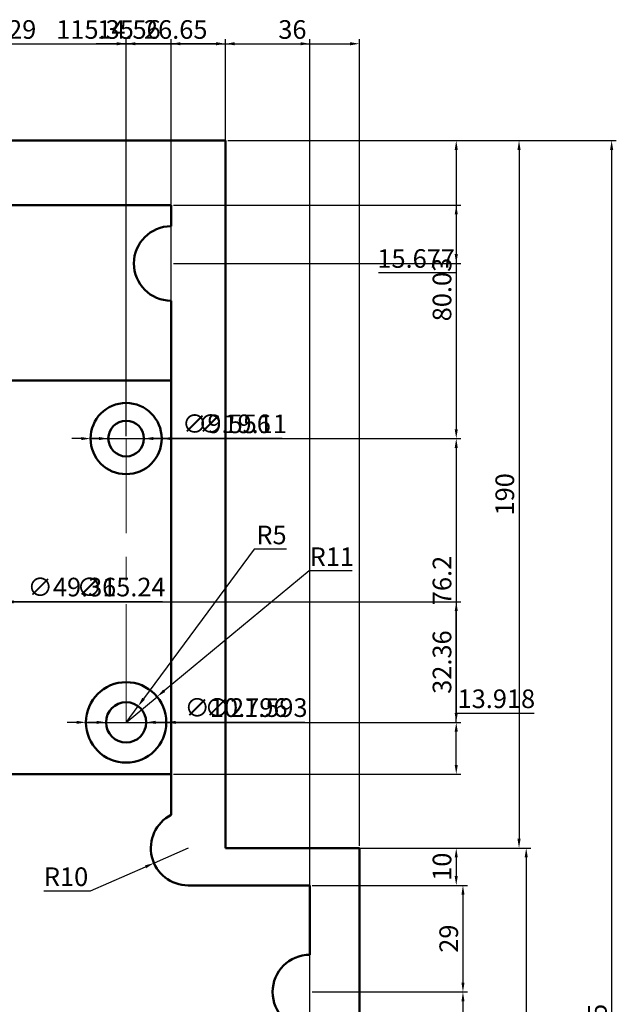
# Model space of a CAD drawing. Units: millimetres. Extents: x 1744 to 2162, y 1763 to 2334.
# Tile 5 of 5: x 1975 to 2135, y 2070 to 2334. Entities that reach past the tile are written whole.
import ezdxf

# ---------------------------------------------------------------- set-up
doc = ezdxf.new("R2010")
doc.units = ezdxf.units.MM
doc.linetypes.add('CENTER', pattern=[50.8, 31.75, -6.35, 6.35, -6.35])
for name, color, linetype, lineweight in [('M-CNTR', 4, 'CENTER', 18), ('M-DIMS', 2, 'Continuous', 25), ('M-OUTL', 7, 'Continuous', 50)]:
    doc.layers.add(name, color=color, linetype=linetype, lineweight=lineweight)
doc.styles.get("Standard").update_dxf_attribs({"font": 'arial.ttf'})
doc.dimstyles.new('ISO-25', dxfattribs={"dimtxt": 5, "dimasz": 2.5, "dimexe": 1.25, "dimexo": 0.625, "dimtad": 1, "dimtoh": 1, "dimdec": 0, "dimtxsty": 'Standard', "dimcen": 2.5, "dimadec": 0, "dimazin": 0, "dimtfac": 1, "dimtdec": 0, "dimtmove": 0, "dimatfit": 3, "dimfxl": 1, "dimarcsym": 0})

# ---------------------------------------------------------------- blocks, each defined once
blk = doc.blocks.new('*D2')
at = {"layer": 'Defpoints', "color": 0, "transparency": 16777216}
for p in [(2029.83, 2301.76), (2035.83, 1826.76), (2133.56, 1826.76)]:
    blk.add_point(p, dxfattribs=at)
at = {"layer": 'M-DIMS', "color": 0, "lineweight": -2, "transparency": 16777216}
for p, q in [((2030.45, 2301.76), (2134.81, 2301.76)), ((2133.56, 2299.26), (2133.56, 1829.26)), ((2036.45, 1826.76), (2134.81, 1826.76))]:
    blk.add_line(p, q, dxfattribs=at)
at = {"layer": 'M-DIMS', "color": 0, "transparency": 16777216}
for points in [[(2133.14, 2299.26), (2133.98, 2299.26), (2133.56, 2301.76)], [(2133.14, 1829.26), (2133.98, 1829.26), (2133.56, 1826.76)]]:
    blk.add_solid(points, dxfattribs=at)
at = {"layer": 'M-DIMS', "color": 0, "transparency": 16777216, "insert": (2130.39, 2064.26), "char_height": 5, "attachment_point": 5, "rotation": 90}
blk.add_mtext('475', dxfattribs=at)
blk = doc.blocks.new('*D3')
at = {"layer": 'Defpoints', "color": 0, "transparency": 16777216}
for p in [(2029.83, 2301.76), (2029.83, 2111.76), (2108.69, 2111.76)]:
    blk.add_point(p, dxfattribs=at)
at = {"layer": 'M-DIMS', "color": 0, "lineweight": -2, "transparency": 16777216}
for p, q in [((2030.45, 2301.76), (2109.94, 2301.76)), ((2108.69, 2299.26), (2108.69, 2114.26)), ((2030.45, 2111.76), (2109.94, 2111.76))]:
    blk.add_line(p, q, dxfattribs=at)
at = {"layer": 'M-DIMS', "color": 0, "transparency": 16777216}
for points in [[(2108.27, 2299.26), (2109.1, 2299.26), (2108.69, 2301.76)], [(2108.27, 2114.26), (2109.1, 2114.26), (2108.69, 2111.76)]]:
    blk.add_solid(points, dxfattribs=at)
at = {"layer": 'M-DIMS', "color": 0, "transparency": 16777216, "insert": (2105.51, 2206.76), "char_height": 5, "attachment_point": 5, "rotation": 90}
blk.add_mtext('190', dxfattribs=at)
blk = doc.blocks.new('*D4')
at = {"layer": 'Defpoints', "color": 0, "transparency": 16777216}
for p in [(2065.83, 2111.76), (2065.83, 1844.08), (2110.62, 1844.08)]:
    blk.add_point(p, dxfattribs=at)
at = {"layer": 'M-DIMS', "color": 0, "lineweight": -2, "transparency": 16777216}
for p, q in [((2066.45, 2111.76), (2111.87, 2111.76)), ((2110.62, 2109.26), (2110.62, 1846.58)), ((2066.45, 1844.08), (2111.87, 1844.08))]:
    blk.add_line(p, q, dxfattribs=at)
at = {"layer": 'M-DIMS', "color": 0, "transparency": 16777216}
for points in [[(2110.2, 2109.26), (2111.04, 2109.26), (2110.62, 2111.76)], [(2110.2, 1846.58), (2111.04, 1846.58), (2110.62, 1844.08)]]:
    blk.add_solid(points, dxfattribs=at)
at = {"layer": 'M-DIMS', "color": 0, "transparency": 16777216, "insert": (2107.44, 1977.92), "char_height": 5, "attachment_point": 5, "rotation": 90}
blk.add_mtext('268', dxfattribs=at)
blk = doc.blocks.new('*D21')
at = {"layer": 'Defpoints', "color": 0, "transparency": 16777216}
for p in [(2019.83, 2111.76), (2010.67, 2107.74)]:
    blk.add_point(p, dxfattribs=at)
at = {"layer": 'M-DIMS', "color": 0, "lineweight": -2, "transparency": 16777216}
for p, q in [((2019.83, 2111.76), (2010.67, 2107.74)), ((1993.64, 2100.25), (2008.38, 2106.73)), ((1981.09, 2100.25), (1993.64, 2100.25))]:
    blk.add_line(p, q, dxfattribs=at)
at = {"layer": 'M-DIMS', "color": 0, "transparency": 16777216}
blk.add_solid([(2008.21, 2107.11), (2008.55, 2106.35), (2010.67, 2107.74)], dxfattribs=at)
at = {"layer": 'M-DIMS', "color": 0, "transparency": 16777216, "insert": (1987.05, 2103.43), "char_height": 5, "attachment_point": 5}
blk.add_mtext('R10', dxfattribs=at)
blk = doc.blocks.new('*D22')
at = {"layer": 'Defpoints', "color": 0, "transparency": 16777216}
for p in [(2011.49, 2152.42), (2003.18, 2145.53)]:
    blk.add_point(p, dxfattribs=at)
at = {"layer": 'M-DIMS', "color": 0, "lineweight": -2, "transparency": 16777216}
for p, q in [((2052.3, 2186.23), (2013.42, 2154.01)), ((2063.91, 2186.23), (2052.3, 2186.23)), ((2003.18, 2145.53), (2011.49, 2152.42))]:
    blk.add_line(p, q, dxfattribs=at)
at = {"layer": 'M-DIMS', "color": 0, "transparency": 16777216}
blk.add_solid([(2013.15, 2154.33), (2013.68, 2153.69), (2011.49, 2152.42)], dxfattribs=at)
at = {"layer": 'M-DIMS', "color": 0, "transparency": 16777216, "insert": (2058.42, 2189.36), "char_height": 5, "attachment_point": 5}
blk.add_mtext('R11', dxfattribs=at)
blk = doc.blocks.new('*D23')
at = {"layer": 'Defpoints', "color": 0, "transparency": 16777216}
for p in [(2006.39, 2149.87), (2003.18, 2145.53)]:
    blk.add_point(p, dxfattribs=at)
at = {"layer": 'M-DIMS', "color": 0, "lineweight": -2, "transparency": 16777216}
for p, q in [((2037.53, 2192.04), (2007.87, 2151.88)), ((2046.26, 2192.04), (2037.53, 2192.04)), ((2003.18, 2145.53), (2006.39, 2149.87))]:
    blk.add_line(p, q, dxfattribs=at)
at = {"layer": 'M-DIMS', "color": 0, "transparency": 16777216}
blk.add_solid([(2007.54, 2152.13), (2008.21, 2151.63), (2006.39, 2149.87)], dxfattribs=at)
at = {"layer": 'M-DIMS', "color": 0, "transparency": 16777216, "insert": (2042.21, 2195.21), "char_height": 5, "attachment_point": 5}
blk.add_mtext('R5', dxfattribs=at)
blk = doc.blocks.new('*D24')
at = {"layer": 'Defpoints', "color": 0, "transparency": 16777216}
for p in [(2052.51, 2101.76), (2052.51, 2073.12), (2093.63, 2073.12)]:
    blk.add_point(p, dxfattribs=at)
at = {"layer": 'M-DIMS', "color": 0, "lineweight": -2, "transparency": 16777216}
for p, q in [((2053.13, 2101.76), (2094.88, 2101.76)), ((2093.63, 2099.26), (2093.63, 2075.62)), ((2053.13, 2073.12), (2094.88, 2073.12))]:
    blk.add_line(p, q, dxfattribs=at)
at = {"layer": 'M-DIMS', "color": 0, "transparency": 16777216}
for points in [[(2093.22, 2099.26), (2094.05, 2099.26), (2093.63, 2101.76)], [(2093.22, 2075.62), (2094.05, 2075.62), (2093.63, 2073.12)]]:
    blk.add_solid(points, dxfattribs=at)
at = {"layer": 'M-DIMS', "color": 0, "transparency": 16777216, "insert": (2090.46, 2087.44), "char_height": 5, "attachment_point": 5, "rotation": 90}
blk.add_mtext('29', dxfattribs=at)
blk = doc.blocks.new('*D25')
at = {"layer": 'Defpoints', "color": 0, "transparency": 16777216}
for p in [(2052.51, 2073.12), (2052.51, 1966.98), (2093.63, 1966.98)]:
    blk.add_point(p, dxfattribs=at)
at = {"layer": 'M-DIMS', "color": 0, "lineweight": -2, "transparency": 16777216}
for p, q in [((2053.13, 2073.12), (2094.88, 2073.12)), ((2093.63, 2070.62), (2093.63, 1969.48)), ((2053.13, 1966.98), (2094.88, 1966.98))]:
    blk.add_line(p, q, dxfattribs=at)
at = {"layer": 'M-DIMS', "color": 0, "transparency": 16777216}
for points in [[(2093.22, 2070.62), (2094.05, 2070.62), (2093.63, 2073.12)], [(2093.22, 1969.48), (2094.05, 1969.48), (2093.63, 1966.98)]]:
    blk.add_solid(points, dxfattribs=at)
at = {"layer": 'M-DIMS', "color": 0, "transparency": 16777216, "insert": (2090.46, 2020.05), "char_height": 5, "attachment_point": 5, "rotation": 90}
blk.add_mtext('106', dxfattribs=at)
blk = doc.blocks.new('*D29')
at = {"layer": 'Defpoints', "color": 0, "transparency": 16777216}
for p in [(2052.51, 2327.76), (2052.51, 1966.98), (1937.15, 1938.72)]:
    blk.add_point(p, dxfattribs=at)
at = {"layer": 'M-DIMS', "color": 0, "lineweight": -2, "transparency": 16777216}
for p, q in [((1937.15, 1939.34), (1937.15, 2329.01)), ((1939.65, 2327.76), (2050.01, 2327.76)), ((2052.51, 1967.6), (2052.51, 2329.01))]:
    blk.add_line(p, q, dxfattribs=at)
at = {"layer": 'M-DIMS', "color": 0, "transparency": 16777216}
for points in [[(1939.65, 2328.18), (1939.65, 2327.34), (1937.15, 2327.76)], [(2050.01, 2328.18), (2050.01, 2327.34), (2052.51, 2327.76)]]:
    blk.add_solid(points, dxfattribs=at)
at = {"layer": 'M-DIMS', "color": 0, "transparency": 16777216, "insert": (1994.83, 2330.94), "char_height": 5, "attachment_point": 5}
blk.add_mtext('115.35', dxfattribs=at)
blk = doc.blocks.new('*D34')
at = {"layer": 'Defpoints', "color": 0, "transparency": 16777216}
for p in [(2003.18, 2327.76), (2003.18, 2221.73), (1937.89, 2177.89)]:
    blk.add_point(p, dxfattribs=at)
at = {"layer": 'M-DIMS', "color": 0, "lineweight": -2, "transparency": 16777216}
for p, q in [((1937.89, 2178.51), (1937.89, 2329.01)), ((1940.39, 2327.76), (2000.68, 2327.76)), ((2003.18, 2222.36), (2003.18, 2329.01))]:
    blk.add_line(p, q, dxfattribs=at)
at = {"layer": 'M-DIMS', "color": 0, "transparency": 16777216}
for points in [[(1940.39, 2328.18), (1940.39, 2327.34), (1937.89, 2327.76)], [(2000.68, 2328.18), (2000.68, 2327.34), (2003.18, 2327.76)]]:
    blk.add_solid(points, dxfattribs=at)
at = {"layer": 'M-DIMS', "color": 0, "transparency": 16777216, "insert": (1970.53, 2330.94), "char_height": 5, "attachment_point": 5}
blk.add_mtext('65.29', dxfattribs=at)
blk = doc.blocks.new('*D35')
at = {"layer": 'Defpoints', "color": 0, "transparency": 16777216}
for p in [(2003.18, 2327.76), (2029.83, 2301.76), (2003.18, 2221.73)]:
    blk.add_point(p, dxfattribs=at)
at = {"layer": 'M-DIMS', "color": 0, "lineweight": -2, "transparency": 16777216}
for p, q in [((2003.18, 2222.36), (2003.18, 2329.01)), ((2027.33, 2327.76), (2005.68, 2327.76)), ((2029.83, 2302.39), (2029.83, 2329.01))]:
    blk.add_line(p, q, dxfattribs=at)
at = {"layer": 'M-DIMS', "color": 0, "transparency": 16777216}
for points in [[(2005.68, 2328.18), (2005.68, 2327.34), (2003.18, 2327.76)], [(2027.33, 2328.18), (2027.33, 2327.34), (2029.83, 2327.76)]]:
    blk.add_solid(points, dxfattribs=at)
at = {"layer": 'M-DIMS', "color": 0, "transparency": 16777216, "insert": (2016.5, 2330.94), "char_height": 5, "attachment_point": 5}
blk.add_mtext('26.65', dxfattribs=at)
blk = doc.blocks.new('*D40')
at = {"layer": 'Defpoints', "color": 0, "transparency": 16777216}
for p in [(1937.89, 2177.89), (2091.83, 2177.89), (2003.18, 2145.53)]:
    blk.add_point(p, dxfattribs=at)
at = {"layer": 'M-DIMS', "color": 0, "lineweight": -2, "transparency": 16777216}
for p, q in [((1938.51, 2177.89), (2093.08, 2177.89)), ((2091.83, 2148.03), (2091.83, 2175.39)), ((2003.8, 2145.53), (2093.08, 2145.53))]:
    blk.add_line(p, q, dxfattribs=at)
at = {"layer": 'M-DIMS', "color": 0, "transparency": 16777216}
for points in [[(2091.41, 2175.39), (2092.24, 2175.39), (2091.83, 2177.89)], [(2091.41, 2148.03), (2092.24, 2148.03), (2091.83, 2145.53)]]:
    blk.add_solid(points, dxfattribs=at)
at = {"layer": 'M-DIMS', "color": 0, "transparency": 16777216, "insert": (2088.65, 2161.71), "char_height": 5, "attachment_point": 5, "rotation": 90}
blk.add_mtext('32.36', dxfattribs=at)
blk = doc.blocks.new('*D43')
at = {"layer": 'Defpoints', "color": 0, "transparency": 16777216}
for p in [(2029.83, 2301.76), (2003.18, 2221.73), (2091.83, 2221.73)]:
    blk.add_point(p, dxfattribs=at)
at = {"layer": 'M-DIMS', "color": 0, "lineweight": -2, "transparency": 16777216}
for p, q in [((2030.45, 2301.76), (2093.08, 2301.76)), ((2091.83, 2299.26), (2091.83, 2224.23)), ((2003.8, 2221.73), (2093.08, 2221.73))]:
    blk.add_line(p, q, dxfattribs=at)
at = {"layer": 'M-DIMS', "color": 0, "transparency": 16777216}
for points in [[(2091.41, 2299.26), (2092.24, 2299.26), (2091.83, 2301.76)], [(2091.41, 2224.23), (2092.24, 2224.23), (2091.83, 2221.73)]]:
    blk.add_solid(points, dxfattribs=at)
at = {"layer": 'M-DIMS', "color": 0, "transparency": 16777216, "insert": (2088.65, 2261.75), "char_height": 5, "attachment_point": 5, "rotation": 90}
blk.add_mtext('80.03', dxfattribs=at)
blk = doc.blocks.new('*D44')
at = {"layer": 'Defpoints', "color": 0, "transparency": 16777216}
for p in [(2003.18, 2221.73), (2003.18, 2145.53), (2091.83, 2145.53)]:
    blk.add_point(p, dxfattribs=at)
at = {"layer": 'M-DIMS', "color": 0, "lineweight": -2, "transparency": 16777216}
for p, q in [((2003.8, 2221.73), (2093.08, 2221.73)), ((2091.83, 2219.23), (2091.83, 2148.03)), ((2003.8, 2145.53), (2093.08, 2145.53))]:
    blk.add_line(p, q, dxfattribs=at)
at = {"layer": 'M-DIMS', "color": 0, "transparency": 16777216}
for points in [[(2091.41, 2219.23), (2092.24, 2219.23), (2091.83, 2221.73)], [(2091.41, 2148.03), (2092.24, 2148.03), (2091.83, 2145.53)]]:
    blk.add_solid(points, dxfattribs=at)
at = {"layer": 'M-DIMS', "color": 0, "transparency": 16777216, "insert": (2088.65, 2183.63), "char_height": 5, "attachment_point": 5, "rotation": 90}
blk.add_mtext('76.2', dxfattribs=at)
blk = doc.blocks.new('*D45')
at = {"layer": 'Defpoints', "color": 0, "transparency": 16777216}
for p in [(2065.83, 2327.76), (2029.83, 2111.76), (2065.83, 2111.76)]:
    blk.add_point(p, dxfattribs=at)
at = {"layer": 'M-DIMS', "color": 0, "lineweight": -2, "transparency": 16777216}
for p, q in [((2029.83, 2112.39), (2029.83, 2329.01)), ((2032.33, 2327.76), (2063.33, 2327.76)), ((2065.83, 2112.39), (2065.83, 2329.01))]:
    blk.add_line(p, q, dxfattribs=at)
at = {"layer": 'M-DIMS', "color": 0, "transparency": 16777216}
for points in [[(2032.33, 2328.18), (2032.33, 2327.34), (2029.83, 2327.76)], [(2063.33, 2328.18), (2063.33, 2327.34), (2065.83, 2327.76)]]:
    blk.add_solid(points, dxfattribs=at)
at = {"layer": 'M-DIMS', "color": 0, "transparency": 16777216, "insert": (2047.83, 2330.94), "char_height": 5, "attachment_point": 5}
blk.add_mtext('36', dxfattribs=at)
blk = doc.blocks.new('*D46')
at = {"layer": 'Defpoints', "color": 0, "transparency": 16777216}
for p in [(2052.51, 2327.76), (1861.12, 1859.18), (2052.51, 1857.29)]:
    blk.add_point(p, dxfattribs=at)
at = {"layer": 'M-DIMS', "color": 0, "lineweight": -2, "transparency": 16777216}
for p, q in [((1861.12, 1859.81), (1861.12, 2329.01)), ((1863.62, 2327.76), (2050.01, 2327.76)), ((2052.51, 1857.91), (2052.51, 2329.01))]:
    blk.add_line(p, q, dxfattribs=at)
at = {"layer": 'M-DIMS', "color": 0, "transparency": 16777216}
for points in [[(1863.62, 2328.18), (1863.62, 2327.34), (1861.12, 2327.76)], [(2050.01, 2328.18), (2050.01, 2327.34), (2052.51, 2327.76)]]:
    blk.add_solid(points, dxfattribs=at)
at = {"layer": 'M-DIMS', "color": 0, "transparency": 16777216, "insert": (1956.82, 2330.94), "char_height": 5, "attachment_point": 5}
blk.add_mtext('191.4', dxfattribs=at)
blk = doc.blocks.new('*D56')
at = {"layer": 'Defpoints', "color": 0, "transparency": 16777216}
for p in [(2015.26, 2327.76), (2015.26, 2120.66), (2029.83, 2111.76)]:
    blk.add_point(p, dxfattribs=at)
at = {"layer": 'M-DIMS', "color": 0, "lineweight": -2, "transparency": 16777216}
for p, q in [((2015.26, 2327.76), (1995.12, 2327.76)), ((2015.26, 2121.28), (2015.26, 2329.01)), ((2027.33, 2327.76), (2017.76, 2327.76)), ((2029.83, 2112.39), (2029.83, 2329.01))]:
    blk.add_line(p, q, dxfattribs=at)
at = {"layer": 'M-DIMS', "color": 0, "transparency": 16777216}
for points in [[(2017.76, 2328.18), (2017.76, 2327.34), (2015.26, 2327.76)], [(2027.33, 2328.18), (2027.33, 2327.34), (2029.83, 2327.76)]]:
    blk.add_solid(points, dxfattribs=at)
at = {"layer": 'M-DIMS', "color": 0, "transparency": 16777216, "insert": (2003.94, 2330.94), "char_height": 5, "attachment_point": 5}
blk.add_mtext('14.56', dxfattribs=at)
blk = doc.blocks.new('*D57')
at = {"layer": 'Defpoints', "color": 0, "transparency": 16777216}
for p in [(2065.83, 2111.76), (2052.51, 2101.76), (2091.83, 2101.76)]:
    blk.add_point(p, dxfattribs=at)
at = {"layer": 'M-DIMS', "color": 0, "lineweight": -2, "transparency": 16777216}
for p, q in [((2066.45, 2111.76), (2093.08, 2111.76)), ((2091.83, 2109.26), (2091.83, 2104.26)), ((2053.13, 2101.76), (2093.08, 2101.76))]:
    blk.add_line(p, q, dxfattribs=at)
at = {"layer": 'M-DIMS', "color": 0, "transparency": 16777216}
for points in [[(2091.41, 2109.26), (2092.24, 2109.26), (2091.83, 2111.76)], [(2091.41, 2104.26), (2092.24, 2104.26), (2091.83, 2101.76)]]:
    blk.add_solid(points, dxfattribs=at)
at = {"layer": 'M-DIMS', "color": 0, "transparency": 16777216, "insert": (2088.65, 2106.76), "char_height": 5, "attachment_point": 5, "rotation": 90}
blk.add_mtext('10', dxfattribs=at)
blk = doc.blocks.new('*D68')
at = {"layer": 'Defpoints', "color": 0, "transparency": 16777216}
for p in [(2015.26, 2284.44), (2015.26, 2268.76), (2091.83, 2268.76)]:
    blk.add_point(p, dxfattribs=at)
at = {"layer": 'M-DIMS', "color": 0, "lineweight": -2, "transparency": 16777216}
for p, q in [((2015.89, 2284.44), (2093.08, 2284.44)), ((2091.83, 2281.94), (2091.83, 2271.26)), ((2015.89, 2268.76), (2093.08, 2268.76)), ((2091.83, 2268.76), (2091.83, 2266.26)), ((2091.83, 2266.26), (2070.91, 2266.26))]:
    blk.add_line(p, q, dxfattribs=at)
at = {"layer": 'M-DIMS', "color": 0, "transparency": 16777216}
for points in [[(2091.41, 2281.94), (2092.24, 2281.94), (2091.83, 2284.44)], [(2091.41, 2271.26), (2092.24, 2271.26), (2091.83, 2268.76)]]:
    blk.add_solid(points, dxfattribs=at)
at = {"layer": 'M-DIMS', "color": 0, "transparency": 16777216, "insert": (2081.06, 2269.44), "char_height": 5, "attachment_point": 5}
blk.add_mtext('15.677', dxfattribs=at)
blk = doc.blocks.new('*D70')
at = {"layer": 'Defpoints', "color": 0, "transparency": 16777216}
for p in [(2003.18, 2145.53), (2091.83, 2145.53), (2015.26, 2131.61)]:
    blk.add_point(p, dxfattribs=at)
at = {"layer": 'M-DIMS', "color": 0, "lineweight": -2, "transparency": 16777216}
for p, q in [((2091.83, 2145.53), (2091.83, 2148.03)), ((2091.83, 2148.03), (2112.75, 2148.03)), ((2003.8, 2145.53), (2093.08, 2145.53)), ((2091.83, 2134.11), (2091.83, 2143.03)), ((2015.89, 2131.61), (2093.08, 2131.61))]:
    blk.add_line(p, q, dxfattribs=at)
at = {"layer": 'M-DIMS', "color": 0, "transparency": 16777216}
for points in [[(2091.41, 2143.03), (2092.24, 2143.03), (2091.83, 2145.53)], [(2091.41, 2134.11), (2092.24, 2134.11), (2091.83, 2131.61)]]:
    blk.add_solid(points, dxfattribs=at)
at = {"layer": 'M-DIMS', "color": 0, "transparency": 16777216, "insert": (2102.6, 2151.21), "char_height": 5, "attachment_point": 5}
blk.add_mtext('13.918', dxfattribs=at)
blk = doc.blocks.new('*D72')
at = {"layer": 'Defpoints', "color": 0, "transparency": 16777216}
for p in [(1993.62, 2221.73), (2012.73, 2221.73)]:
    blk.add_point(p, dxfattribs=at)
at = {"layer": 'M-DIMS', "color": 0, "lineweight": -2, "transparency": 16777216}
for p, q in [((1991.12, 2221.73), (1988.62, 2221.73)), ((1993.62, 2221.73), (2012.73, 2221.73)), ((2023.12, 2221.73), (2015.23, 2221.73)), ((2045.09, 2221.73), (2023.12, 2221.73))]:
    blk.add_line(p, q, dxfattribs=at)
at = {"layer": 'M-DIMS', "color": 0, "transparency": 16777216}
for points in [[(1991.12, 2222.15), (1991.12, 2221.32), (1993.62, 2221.73)], [(2015.23, 2222.15), (2015.23, 2221.32), (2012.73, 2221.73)]]:
    blk.add_solid(points, dxfattribs=at)
at = {"layer": 'M-DIMS', "color": 0, "transparency": 16777216, "insert": (2034.42, 2225.05), "char_height": 5, "attachment_point": 5}
blk.add_mtext('∅19.11', dxfattribs=at)
blk = doc.blocks.new('*D73')
at = {"layer": 'Defpoints', "color": 0, "transparency": 16777216}
for p in [(1998.4, 2221.73), (2007.96, 2221.73)]:
    blk.add_point(p, dxfattribs=at)
at = {"layer": 'M-DIMS', "color": 0, "lineweight": -2, "transparency": 16777216}
for p, q in [((1995.9, 2221.73), (1993.4, 2221.73)), ((1998.4, 2221.73), (2007.96, 2221.73)), ((2018.34, 2221.73), (2010.46, 2221.73)), ((2041.28, 2221.73), (2018.34, 2221.73))]:
    blk.add_line(p, q, dxfattribs=at)
at = {"layer": 'M-DIMS', "color": 0, "transparency": 16777216}
for points in [[(1995.9, 2222.15), (1995.9, 2221.32), (1998.4, 2221.73)], [(2010.46, 2222.15), (2010.46, 2221.32), (2007.96, 2221.73)]]:
    blk.add_solid(points, dxfattribs=at)
at = {"layer": 'M-DIMS', "color": 0, "transparency": 16777216, "insert": (2030.12, 2225.05), "char_height": 5, "attachment_point": 5}
blk.add_mtext('∅9.556', dxfattribs=at)
blk = doc.blocks.new('*D79')
at = {"layer": 'Defpoints', "color": 0, "transparency": 16777216}
for p in [(1905.27, 2177.89), (1970.5, 2177.89)]:
    blk.add_point(p, dxfattribs=at)
at = {"layer": 'M-DIMS', "color": 0, "lineweight": -2, "transparency": 16777216}
for p, q in [((1902.77, 2177.89), (1900.27, 2177.89)), ((1905.27, 2177.89), (1970.5, 2177.89)), ((1990.07, 2177.89), (1973, 2177.89)), ((2012.99, 2177.89), (1990.07, 2177.89))]:
    blk.add_line(p, q, dxfattribs=at)
at = {"layer": 'M-DIMS', "color": 0, "transparency": 16777216}
for points in [[(1902.77, 2178.3), (1902.77, 2177.47), (1905.27, 2177.89)], [(1973, 2178.3), (1973, 2177.47), (1970.5, 2177.89)]]:
    blk.add_solid(points, dxfattribs=at)
at = {"layer": 'M-DIMS', "color": 0, "transparency": 16777216, "insert": (2001.84, 2181.21), "char_height": 5, "attachment_point": 5}
blk.add_mtext('∅65.24', dxfattribs=at)
blk = doc.blocks.new('*D82')
at = {"layer": 'Defpoints', "color": 0, "transparency": 16777216}
for p in [(1913.23, 2177.89), (1962.54, 2177.89)]:
    blk.add_point(p, dxfattribs=at)
at = {"layer": 'M-DIMS', "color": 0, "lineweight": -2, "transparency": 16777216}
for p, q in [((1910.73, 2177.89), (1908.23, 2177.89)), ((1913.23, 2177.89), (1962.54, 2177.89)), ((1977.34, 2177.89), (1965.04, 2177.89)), ((1999.31, 2177.89), (1977.34, 2177.89))]:
    blk.add_line(p, q, dxfattribs=at)
at = {"layer": 'M-DIMS', "color": 0, "transparency": 16777216}
for points in [[(1910.73, 2178.3), (1910.73, 2177.47), (1913.23, 2177.89)], [(1965.04, 2178.3), (1965.04, 2177.47), (1962.54, 2177.89)]]:
    blk.add_solid(points, dxfattribs=at)
at = {"layer": 'M-DIMS', "color": 0, "transparency": 16777216, "insert": (1988.63, 2181.21), "char_height": 5, "attachment_point": 5}
blk.add_mtext('∅49.31', dxfattribs=at)
blk = doc.blocks.new('*D87')
at = {"layer": 'Defpoints', "color": 0, "transparency": 16777216}
for p in [(1992.38, 2145.53), (2013.97, 2145.53)]:
    blk.add_point(p, dxfattribs=at)
at = {"layer": 'M-DIMS', "color": 0, "lineweight": -2, "transparency": 16777216}
for p, q in [((1989.88, 2145.53), (1987.38, 2145.53)), ((1992.38, 2145.53), (2013.97, 2145.53)), ((2024.36, 2145.53), (2016.47, 2145.53)), ((2051.18, 2145.53), (2024.36, 2145.53))]:
    blk.add_line(p, q, dxfattribs=at)
at = {"layer": 'M-DIMS', "color": 0, "transparency": 16777216}
for points in [[(1989.88, 2145.94), (1989.88, 2145.11), (1992.38, 2145.53)], [(2016.47, 2145.94), (2016.47, 2145.11), (2013.97, 2145.53)]]:
    blk.add_solid(points, dxfattribs=at)
at = {"layer": 'M-DIMS', "color": 0, "transparency": 16777216, "insert": (2038.08, 2148.84), "char_height": 5, "attachment_point": 5}
blk.add_mtext('∅21.593', dxfattribs=at)
blk = doc.blocks.new('*D90')
at = {"layer": 'Defpoints', "color": 0, "transparency": 16777216}
for p in [(1997.78, 2145.53), (2008.58, 2145.53)]:
    blk.add_point(p, dxfattribs=at)
at = {"layer": 'M-DIMS', "color": 0, "lineweight": -2, "transparency": 16777216}
for p, q in [((1995.28, 2145.53), (1992.78, 2145.53)), ((1997.78, 2145.53), (2008.58, 2145.53)), ((2018.96, 2145.53), (2011.08, 2145.53)), ((2045.78, 2145.53), (2018.96, 2145.53))]:
    blk.add_line(p, q, dxfattribs=at)
at = {"layer": 'M-DIMS', "color": 0, "transparency": 16777216}
for points in [[(1995.28, 2145.94), (1995.28, 2145.11), (1997.78, 2145.53)], [(2011.08, 2145.94), (2011.08, 2145.11), (2008.58, 2145.53)]]:
    blk.add_solid(points, dxfattribs=at)
at = {"layer": 'M-DIMS', "color": 0, "transparency": 16777216, "insert": (2032.68, 2148.84), "char_height": 5, "attachment_point": 5}
blk.add_mtext('∅10.796', dxfattribs=at)

msp = doc.modelspace()

# ---------------------------------------------------------------- linework, layer by layer
at = {"layer": 'M-CNTR'}
msp.add_line((2003.178, 2145.5271), (2003.178, 2221.7343), dxfattribs=at)
at = {"layer": 'M-OUTL'}
for p, q in [((1845.8255, 2301.7604), (2029.8255, 2301.7604)), ((2029.8255, 2301.7604), (2029.8255, 2111.7604)), ((2029.8255, 2301.7604), (2029.8255, 2268.7604)), ((1970.6942, 2284.4372), (2015.2647, 2284.4372)), ((2015.2647, 2284.4372), (2015.2647, 2278.7604)), ((2015.2647, 2258.7604), (2015.2647, 2120.6598)), ((2015.2647, 2237.3582), (1925.3972, 2237.3582)), ((1930.1843, 2131.6094), (2015.2647, 2131.6094)), ((2029.8255, 2111.7604), (2065.8255, 2111.7604)), ((2065.8255, 1844.0809), (2065.8255, 2111.7604)), ((2019.8255, 2101.7604), (2052.5068, 2101.7604)), ((2052.5068, 2096.9169), (2052.5068, 2101.7604)), ((2052.5068, 2083.1218), (2052.5068, 2096.9169))]:
    msp.add_line(p, q, dxfattribs=at)
for centre, radius in [((2003.178, 2221.7343), 9.5558), ((2003.178, 2221.7343), 4.7779), ((2003.178, 2145.5271), 10.7964), ((2003.178, 2145.5271), 5.3982)]:
    msp.add_circle(centre, radius, dxfattribs=at)
for centre, start in [((2015.2647, 2268.7604), 90), ((2019.8255, 2111.7604), 117.134434), ((2052.5068, 2073.1218), 90)]:
    msp.add_arc(centre, 10, start, 270, dxfattribs=at)

# ---------------------------------------------------------------- dimensions: what is measured, and where the dimension line sits
at = {"layer": 'M-DIMS'}
for base, p1, p2, override, picture, middle in [((2052.5068, 2327.7604), (1861.1237, 1859.184), (2052.5068, 1857.2889), {"dimdec": 1, "dimlfac": 1, "dimrnd": 0, "dimzin": 0, "dimdsep": 46, "dimlunit": 2}, '*D46', (1956.8153, 2330.9382)), ((2052.5068, 2327.7604), (1937.1543, 1938.7171), (2052.5068, 1966.9753), {"dimdec": 2, "dimlfac": 1, "dimrnd": 0, "dimzin": 0, "dimdsep": 46, "dimlunit": 2}, '*D29', (1994.8306, 2330.9399)), ((2003.178, 2327.7604), (1937.8856, 2177.888), (2003.178, 2221.7343), {"dimdec": 2, "dimlfac": 1, "dimrnd": 0, "dimzin": 0, "dimdsep": 46, "dimlunit": 2}, '*D34', (1970.5318, 2330.9382)), ((2015.2647, 2327.7604), (2029.8255, 2111.7604), (2015.2647, 2120.6598), {"dimdec": 2, "dimlfac": 1, "dimrnd": 0, "dimzin": 0, "dimdsep": 46, "dimlunit": 2}, '*D56', (2003.9405, 2330.9382)), ((2003.178, 2327.7604), (2029.8255, 2301.7604), (2003.178, 2221.7343), {"dimdec": 2, "dimlfac": 1, "dimrnd": 0, "dimzin": 0, "dimdsep": 46, "dimlunit": 2}, '*D35', (2016.5018, 2330.9382)), ((2065.8255, 2327.7604), (2029.8255, 2111.7604), (2065.8255, 2111.7604), {"dimdec": 0, "dimlfac": 1, "dimrnd": 0, "dimzin": 0, "dimdsep": 46, "dimlunit": 2}, '*D45', (2047.8255, 2330.9399))]:
    dim = msp.add_linear_dim(base=base, p1=p1, p2=p2, dimstyle='ISO-25', override=override, dxfattribs=at)
    dim.commit()
    dim.dimension.update_dxf_attribs({"geometry": picture, "text_midpoint": middle})
for base, p1, p2, override, picture, middle in [((2091.8255, 2221.7343), (2029.8255, 2301.7604), (2003.178, 2221.7343), {"dimdec": 2, "dimlfac": 1, "dimrnd": 0, "dimzin": 0, "dimdsep": 46, "dimlunit": 2}, '*D43', (2088.6459, 2261.7473)), ((2133.5602, 1826.7604), (2029.8255, 2301.7604), (2035.8255, 1826.7604), {"dimclrd": 0, "dimclre": 0, "dimclrt": 0}, '*D2', (2130.3925, 2064.2604)), ((2108.686, 2111.7604), (2029.8255, 2301.7604), (2029.8255, 2111.7604), {"dimclrd": 0, "dimclre": 0, "dimclrt": 0}, '*D3', (2105.5081, 2206.7604)), ((2091.8255, 2268.7604), (2015.2647, 2284.4372), (2015.2647, 2268.7604), {"dimdec": 3, "dimlfac": 1, "dimrnd": 0, "dimzin": 0, "dimdsep": 46, "dimlunit": 2}, '*D68', (2081.0572, 2269.4382)), ((2091.8255, 2145.5271), (2003.178, 2221.7343), (2003.178, 2145.5271), {"dimdec": 1, "dimlfac": 1, "dimrnd": 0, "dimzin": 0, "dimdsep": 46, "dimlunit": 2}, '*D44', (2088.6476, 2183.6307)), ((2091.8255, 2177.888), (2003.178, 2145.5271), (1937.8856, 2177.888), {"dimdec": 2, "dimlfac": 1, "dimrnd": 0, "dimzin": 0, "dimdsep": 46, "dimlunit": 2}, '*D40', (2088.6459, 2161.7076)), ((2091.8255, 2145.5271), (2015.2647, 2131.6094), (2003.178, 2145.5271), {"dimdec": 3, "dimlfac": 1, "dimrnd": 0, "dimzin": 0, "dimdsep": 46, "dimlunit": 2}, '*D70', (2102.5988, 2151.2067)), ((2091.8255, 2101.7604), (2065.8255, 2111.7604), (2052.5068, 2101.7604), {"dimdec": 0, "dimlfac": 1, "dimrnd": 0, "dimzin": 0, "dimdsep": 46, "dimlunit": 2}, '*D57', (2088.6476, 2106.7604)), ((2110.6209, 1844.0809), (2065.8255, 2111.7604), (2065.8255, 1844.0809), {"dimclrd": 0, "dimclre": 0, "dimclrt": 0}, '*D4', (2107.4431, 1977.9206)), ((2093.6333, 2073.1218), (2052.5068, 2101.7604), (2052.5068, 2073.1218), {"dimclrd": 0, "dimclre": 0, "dimclrt": 0}, '*D24', (2090.4554, 2087.4411)), ((2093.6333, 1966.9753), (2052.5068, 2073.1218), (2052.5068, 1966.9753), {"dimclrd": 0, "dimclre": 0, "dimclrt": 0}, '*D25', (2090.4554, 2020.0486))]:
    dim = msp.add_linear_dim(base=base, p1=p1, p2=p2, angle=90, dimstyle='ISO-25', override=override, dxfattribs=at)
    dim.commit()
    dim.dimension.update_dxf_attribs({"geometry": picture, "text_midpoint": middle})
for p1, p2, override, picture, middle in [((1993.6222, 2221.7346), (2012.7339, 2221.734), {"dimdec": 2, "dimlfac": 1, "dimrnd": 0, "dimzin": 0, "dimdsep": 46, "dimlunit": 2}, '*D72', (2023.1193, 2221.7337)), ((1998.4001, 2221.7346), (2007.9559, 2221.734), {"dimdec": 3, "dimlfac": 1, "dimrnd": 0, "dimzin": 0, "dimdsep": 46, "dimlunit": 2}, '*D73', (2018.3413, 2221.7333)), ((1905.268, 2177.8879), (1970.5033, 2177.888), {"dimdec": 2, "dimlfac": 1, "dimrnd": 0, "dimzin": 0, "dimdsep": 46, "dimlunit": 2}, '*D79', (1990.0739, 2177.888)), ((1913.2298, 2177.8879), (1962.5415, 2177.888), {"dimdec": 2, "dimlfac": 1, "dimrnd": 0, "dimzin": 0, "dimdsep": 46, "dimlunit": 2}, '*D82', (1977.335, 2177.888)), ((1997.7798, 2145.5273), (2008.5762, 2145.527), {"dimdec": 3, "dimlfac": 1, "dimrnd": 0, "dimzin": 0, "dimdsep": 46, "dimlunit": 2}, '*D90', (2018.9616, 2145.5267))]:
    dim = msp.add_diameter_dim_2p(p1=p1, p2=p2, dimstyle='ISO-25', override=override, dxfattribs=at)
    dim.commit()
    dim.dimension.update_dxf_attribs({"geometry": picture, "text_midpoint": middle, "dimtype": 163})
for center, mpoint, picture, middle in [((2003.178, 2145.5271), (2006.3852, 2149.8693), '*D23', (2042.209, 2192.0421)), ((2003.178, 2145.5271), (2011.4918, 2152.4151), '*D22', (2058.4208, 2186.2284)), ((2019.8255, 2111.7604), (2010.671, 2107.7361), '*D21', (1987.0525, 2100.2506))]:
    dim = msp.add_radius_dim(center=center, mpoint=mpoint, dimstyle='ISO-25', override={"dimclrd": 0, "dimclre": 0, "dimclrt": 0}, dxfattribs=at)
    dim.commit()
    dim.dimension.update_dxf_attribs({"geometry": picture, "text_midpoint": middle, "dimtype": 164})
dim = msp.add_diameter_dim_2p(p1=(1992.3817, 2145.5273), p2=(2013.9744, 2145.527), dimstyle='ISO-25', override={"dimdec": 3, "dimlfac": 1, "dimrnd": 0, "dimzin": 0, "dimdsep": 46, "dimlunit": 2}, dxfattribs=at)
dim.commit()
dim.dimension.update_dxf_attribs({"geometry": '*D87', "text_midpoint": (2024.3598, 2145.5269)})

doc.saveas('drawing.dxf')
